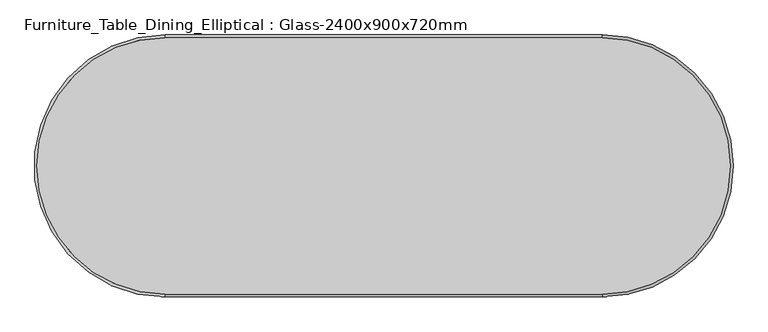
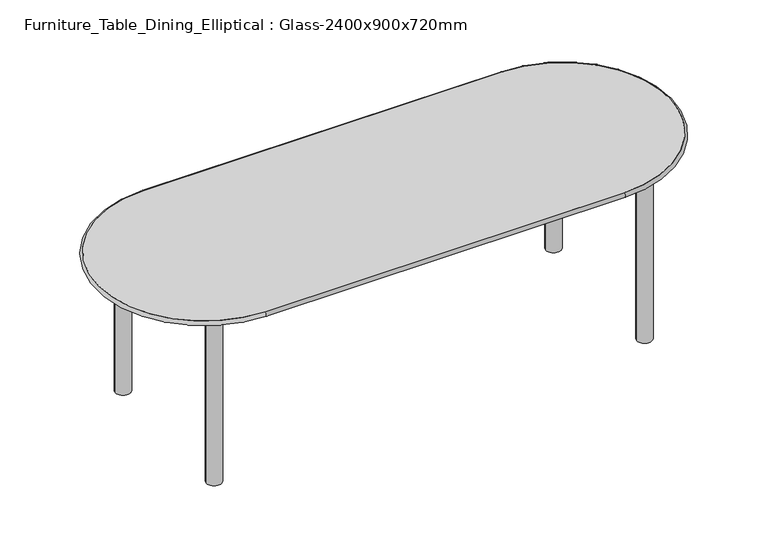
"""IFC4 building model written with IfcOpenShell, lengths in millimetres: furniture geometry, Furniture_Table_Dining_Elliptical : Glass-2400x900x720mm."""

from ifc_helpers import new_model, si_unit, point, frame, frame_2d, origin, origin_with_axes, place, context, project, spatial, polyline, circle_curve, ellipse_curve, trimmed, segment, composite_curve, outline, extrude, source, transform, mapped, element, save
from ifc_brep_helpers import plane_surface, cylinder_surface, revolved_surface, advanced_brep


def furniture_table_dining_elliptical_glass_2400x900x720mm_3aac8a2d(model_context):
    return source(origin(), model_context, "Body", "SolidModel", [
        extrude(outline(composite_curve([segment(polyline([(-1151.8196721, 82.3766393), (348.1803279, 82.3766393)]), True, "CONTINUOUS"), segment(trimmed(circle_curve(frame_2d((348.1803279, -358.0983607)), 440.475), [point((348.1803279, 82.3766393))], [point((788.6553279, -358.0983607))], False, "CARTESIAN"), True, "CONTINUOUS"), segment(trimmed(circle_curve(frame_2d((348.1803279, -358.0983607)), 440.475), [point((788.6553279, -358.0983607))], [point((348.1803279, -798.5733607))], False, "CARTESIAN"), True, "CONTINUOUS"), segment(polyline([(348.1803279, -798.5733607), (-1151.8196721, -798.5733607)]), True, "CONTINUOUS"), segment(trimmed(circle_curve(frame_2d((-1151.8196721, -358.0983607)), 440.475), [point((-1151.8196721, -798.5733607))], [point((-1592.2946721, -358.0983607))], False, "CARTESIAN"), True, "CONTINUOUS"), segment(trimmed(circle_curve(frame_2d((-1151.8196721, -358.0983607)), 440.475), [point((-1592.2946721, -358.0983607))], [point((-1151.8196721, 82.3766393))], False, "CARTESIAN"), True, "CONTINUOUS")], self_intersect=False)), frame((0.0, 0.0, 742.95), z_axis=(0.0, 0.0, 1.0), x_axis=(1.0, 0.0, 0.0)), (0.0, 0.0, 1.0), 19.05),
        extrude(outline(polyline([(516.4553279, -9.6983607), (516.4553279, -706.4983607), (-1320.0946721, -706.4983607), (-1320.0946721, -9.6983607), (516.4553279, -9.6983607)]), holes=[polyline([(497.4053279, -28.7483607), (-1301.0446721, -28.7483607), (-1301.0446721, -687.4483607), (497.4053279, -687.4483607), (497.4053279, -28.7483607)])]), frame((0.0, 0.0, 692.15), z_axis=(0.0, 0.0, 1.0), x_axis=(1.0, 0.0, 0.0)), (0.0, 0.0, 1.0), 50.8),
        extrude(outline(composite_curve([segment(trimmed(circle_curve(frame_2d((-1301.0446721, -28.7483607)), 31.75), [point((-1332.7946721, -28.7483607))], [point((-1269.2946721, -28.7483607))], False, "CARTESIAN"), True, "CONTINUOUS"), segment(trimmed(circle_curve(frame_2d((-1301.0446721, -28.7483607)), 31.75), [point((-1269.2946721, -28.7483607))], [point((-1332.7946721, -28.7483607))], False, "CARTESIAN"), True, "CONTINUOUS")], self_intersect=False)), origin_with_axes(), (0.0, 0.0, 1.0), 742.95),
        extrude(outline(composite_curve([segment(trimmed(circle_curve(frame_2d((-1301.0446721, -687.4483607)), 31.75), [point((-1332.7946721, -687.4483607))], [point((-1269.2946721, -687.4483607))], False, "CARTESIAN"), True, "CONTINUOUS"), segment(trimmed(circle_curve(frame_2d((-1301.0446721, -687.4483607)), 31.75), [point((-1269.2946721, -687.4483607))], [point((-1332.7946721, -687.4483607))], False, "CARTESIAN"), True, "CONTINUOUS")], self_intersect=False)), origin_with_axes(), (0.0, 0.0, 1.0), 742.95),
        extrude(outline(composite_curve([segment(trimmed(circle_curve(frame_2d((497.4053279, -28.7483607)), 31.75), [point((465.6553279, -28.7483607))], [point((529.1553279, -28.7483607))], False, "CARTESIAN"), True, "CONTINUOUS"), segment(trimmed(circle_curve(frame_2d((497.4053279, -28.7483607)), 31.75), [point((529.1553279, -28.7483607))], [point((465.6553279, -28.7483607))], False, "CARTESIAN"), True, "CONTINUOUS")], self_intersect=False)), origin_with_axes(), (0.0, 0.0, 1.0), 742.95),
        extrude(outline(composite_curve([segment(trimmed(circle_curve(frame_2d((497.4053279, -687.4483607)), 31.75), [point((465.6553279, -687.4483607))], [point((529.1553279, -687.4483607))], False, "CARTESIAN"), True, "CONTINUOUS"), segment(trimmed(circle_curve(frame_2d((497.4053279, -687.4483607)), 31.75), [point((529.1553279, -687.4483607))], [point((465.6553279, -687.4483607))], False, "CARTESIAN"), True, "CONTINUOUS")], self_intersect=False)), origin_with_axes(), (0.0, 0.0, 1.0), 742.95),
        advanced_brep(
        [(-1151.8196721, -798.5733607, 762.0), (-1151.8196721, -798.5733607, 742.95), (348.1803279, -798.5733607, 742.95), (348.1803279, -798.5733607, 762.0), (348.1803279, 82.3766393, 762.0), (348.1803279, 82.3766393, 742.95), (-1151.8196721, 82.3766393, 742.95), (-1151.8196721, 82.3766393, 762.0)],
        [
            (0, 1, circle_curve(frame((-1151.8196721, -798.5733607, 752.475), z_axis=(1.0, 0.0, 0.0), x_axis=(0.0, 1.0, 0.0)), 9.525)),
            (1, 2),
            (2, 3, circle_curve(frame((348.1803279, -798.5733607, 752.475), z_axis=(-1.0, 0.0, 0.0), x_axis=(0.0, 1.0, 0.0)), 9.525)),
            (3, 0),
            (1, 0),
            (3, 2),
            (4, 3, circle_curve(frame((348.1803279, -358.0983607, 762.0), z_axis=(0.0, 0.0, -1.0), x_axis=(0.0, -1.0, 0.0)), 440.475)),
            (2, 5, circle_curve(frame((348.1803279, -358.0983607, 742.95), z_axis=(0.0, 0.0, 1.0), x_axis=(0.0, -1.0, 0.0)), 440.475)),
            (5, 4, circle_curve(frame((348.1803279, 82.3766393, 752.475), z_axis=(1.0, 0.0, 0.0), x_axis=(0.0, -1.0, 0.0)), 9.525)),
            (4, 5),
            (5, 6),
            (6, 7, circle_curve(frame((-1151.8196721, 82.3766393, 752.475), z_axis=(1.0, 0.0, 0.0), x_axis=(0.0, -1.0, 0.0)), 9.525)),
            (7, 4),
            (7, 6),
            (0, 7, circle_curve(frame((-1151.8196721, -358.0983607, 762.0), z_axis=(0.0, 0.0, -1.0), x_axis=(0.0, 1.0, 0.0)), 440.475)),
            (6, 1, circle_curve(frame((-1151.8196721, -358.0983607, 742.95), z_axis=(0.0, 0.0, 1.0), x_axis=(0.0, 1.0, 0.0)), 440.475)),
        ],
        [
            cylinder_surface(frame((-1151.8196721, -798.5733607, 752.475), z_axis=(-1.0, 0.0, 0.0), x_axis=(0.0, 1.0, 0.0)), 9.525),
            plane_surface(frame((-1151.8196721, -798.5733607, 762.0), z_axis=(0.0, 1.0, 0.0), x_axis=(1.0, 0.0, 0.0))),
            revolved_surface(trimmed(ellipse_curve(frame((348.1803279, -798.5733607, 752.475), z_axis=(-1.0, 0.0, 0.0), x_axis=(0.0, 1.0, 0.0)), 9.525, 9.525), [point((348.1803279, -798.5733607, 742.95))], [point((348.1803279, -798.5733607, 762.0))], True, "CARTESIAN"), (348.1803279, -358.0983607, 0.0), (0.0, 0.0, 1.0)),
            revolved_surface(polyline([(348.1803279, -798.5733607, 762.0), (348.1803279, -798.5733607, 742.95)]), (348.1803279, -358.0983607, 0.0), (0.0, 0.0, 1.0)),
            cylinder_surface(frame((348.1803279, 82.3766393, 752.475), z_axis=(1.0, 0.0, 0.0), x_axis=(0.0, -1.0, 0.0)), 9.525),
            plane_surface(frame((348.1803279, 82.3766393, 762.0), z_axis=(0.0, -1.0, 0.0), x_axis=(-1.0, 0.0, 0.0))),
            revolved_surface(trimmed(ellipse_curve(frame((-1151.8196721, 82.3766393, 752.475), z_axis=(1.0, 0.0, 0.0), x_axis=(0.0, -1.0, 0.0)), 9.525, 9.525), [point((-1151.8196721, 82.3766393, 742.95))], [point((-1151.8196721, 82.3766393, 762.0))], True, "CARTESIAN"), (-1151.8196721, -358.0983607, 0.0), (0.0, 0.0, 1.0)),
            revolved_surface(polyline([(-1151.8196721, 82.37663930000002, 762.0), (-1151.8196721, 82.37663930000002, 742.95)]), (-1151.8196721, -358.0983607, 0.0), (0.0, 0.0, 1.0)),
        ],
        [
            (0, [[1, 2, 3, 4]]),
            (1, [[5, -4, 6, -2]]),
            (2, [[7, -3, 8, 9]]),
            (3, [[-8, -6, -7, 10]]),
            (4, [[-9, 11, 12, 13]]),
            (5, [[-10, -13, 14, -11]]),
            (6, [[15, -12, 16, -1]]),
            (7, [[-16, -14, -15, -5]]),
        ],
    ),
    ])


if __name__ == "__main__":
    model = new_model("IFC4")
    model_context = context("Model", 3, world=origin())
    ifc_project = project(units=[si_unit("LENGTHUNIT", "METRE", prefix="MILLI")], contexts=[model_context])
    site = spatial("IfcSite", under=ifc_project)
    building = spatial("IfcBuilding", under=site)
    placement = place(None, origin())
    furniture_table_dining_elliptical_glass_2400x900x720mm_shape = furniture_table_dining_elliptical_glass_2400x900x720mm_3aac8a2d(model_context)
    element("IfcFurniture", 1, ObjectType="Furniture_Table_Dining_Elliptical : Glass-2400x900x720mm", at=placement, inside=building, context=model_context, shape_type="MappedRepresentation", body=[
        mapped(furniture_table_dining_elliptical_glass_2400x900x720mm_shape, transform((0.0, 0.0, 0.0), x_axis=(1.0, 0.0, 0.0), y_axis=(0.0, 1.0, 0.0), z_axis=(0.0, 0.0, 1.0))),
    ])
    save(model, "model.ifc")

# Revit data of these elements
# Type "Furniture_Table_Dining_Elliptical : Glass-2400x900x720mm"
#   Keynote = "N"
#   Length = 7' - 10.48819"
#   Width = 2' - 11.43307"
#   Material Base = Metal - Bronze, Light Brush
#   Material Top = Glass - Clear, Grey
#   Default Elevation = 0
# Element 1 (IfcFurniture, "Furniture_Table_Dining_Elliptical : Glass-2400x900x720mm")
#   Materials on its faces: "Metal - Bronze, Light Brush", "Glass - Clear, Grey"
# Materials
#   "Metal - Bronze, Light Brush": class "Metal", colour RGB 113 80 70, transparency 0
#   "Glass - Clear, Grey": class "Glass", colour RGB 252 255 255, transparency 0.64
